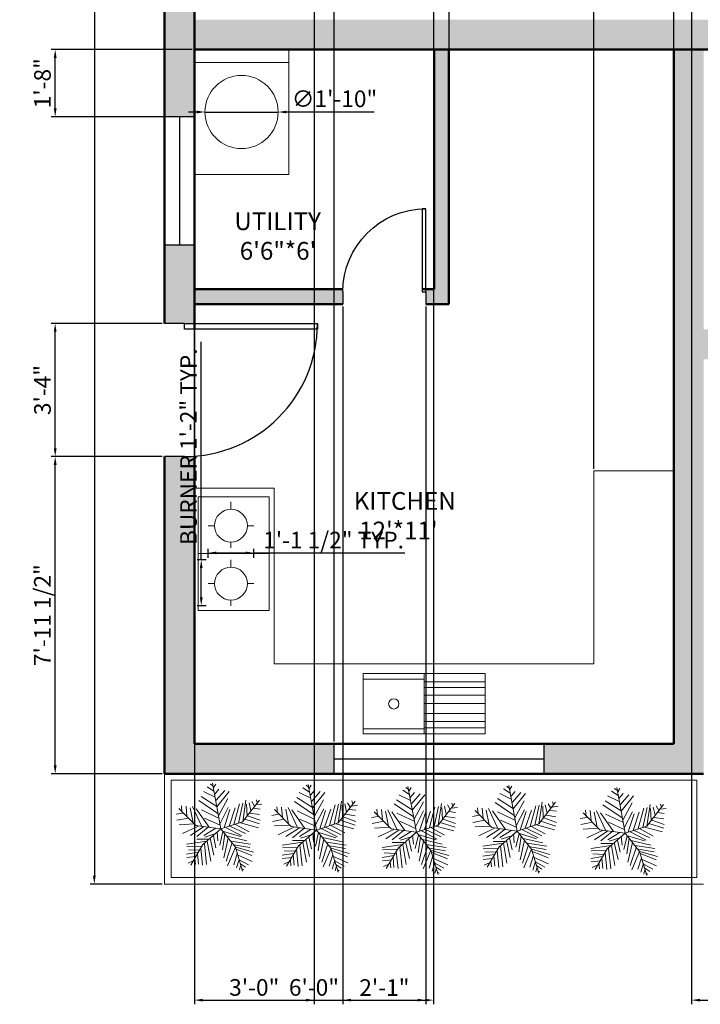
# Model space of a CAD drawing. Units: inches. Extents: x 2152 to 2718, y 1095 to 1798.
# Tile 1 of 5: x 2152 to 2356, y 1098 to 1394. Entities that reach past the tile are written whole.
import ezdxf

# ---------------------------------------------------------------- set-up
doc = ezdxf.new("R2010")
doc.units = ezdxf.units.IN
for name, color, linetype, lineweight in [('A-ANNO-DIMS', 130, 'Continuous', 18), ('A-AREA-IDEN', 130, 'Continuous', 25), ('A-EQPM', 10, 'Continuous', 18), ('A-FLOR-CASE', 10, 'Continuous', 20), ('A-FLOR-FIXT', 10, 'Continuous', 18), ('A-FLOR-STRS', 7, 'Continuous', 25), ('A-WALL-PATT', 210, 'Continuous', 13), ('DOOR', 160, 'Continuous', 25), ('L-PLNT-BEDS', 80, 'Continuous', 18), ('TREE', 80, 'Continuous', 13), ('WALL', 7, 'Continuous', 50), ('WIND', 140, 'Continuous', 25)]:
    doc.layers.add(name, color=color, linetype=linetype, lineweight=lineweight)
doc.styles.get("Standard").update_dxf_attribs({"font": 'arial.ttf'})
doc.dimstyles.new('ISO-25', dxfattribs={"dimtxt": 5, "dimasz": 2.5, "dimexe": 1.25, "dimexo": 0.625, "dimtad": 1, "dimdec": 0, "dimlunit": 4, "dimtxsty": 'Standard', "dimcen": 2.5, "dimadec": 0, "dimazin": 0, "dimtfac": 1, "dimtdec": 0, "dimtmove": 0, "dimatfit": 3, "dimfxl": 1, "dimarcsym": 0})

# ---------------------------------------------------------------- blocks, each defined once
blk = doc.blocks.new('*U6')
for p, q in [((-8.737, 47.138), (-17.069, 52.711)), ((-10.186, 53.64), (-13.084, 55.962)), ((0, 0), (-10.5, 57)), ((-9.099, 51.782), (-6.563, 55.962)), ((-7.65, 43.423), (-2.578, 49.46)), ((-5.114, 28.097), (-24.676, 40.636)), ((-7.288, 39.707), (-21.778, 46.673)), ((-5.839, 35.992), (4.667, 48.067)), ((-5.114, 27.632), (10.463, 46.673)), ((-2.941, 16.486), (8.652, 37.85)), ((-31.5, 4.5), (-52.5, 25.5)), ((-48.585, 21.131), (-49.309, 29.026)), ((-43.513, 28.561), (-42.427, 15.558)), ((-38.442, 26.239), (-34.819, 7.663)), ((-35.544, 28.097), (-24.314, 3.947)), ((-14.533, 2.09), (-30.834, 25.31)), ((-3.665, 19.273), (-27.574, 35.527)), ((-1.129, 6.734), (9.014, 26.704)), ((10.101, 3.483), (17.708, 26.239)), ((16.259, 5.805), (23.142, 31.348)), ((22.055, 7.198), (27.489, 32.277)), ((27, 9), (48, 36)), ((27.127, 9.056), (31.112, 35.992)), ((31.836, 30.883), (32.561, 16.486)), ((35.096, 32.741), (37.27, 22.524)), ((38.719, 34.134), (41.979, 28.561)), ((40.53, 25.775), (48.862, 24.846)), ((43.791, 29.954), (51.036, 30.883)), ((44.153, 36.456), (45.239, 32.741)), ((-47.498, 19.737), (-55.83, 18.344)), ((-40.615, 13.7), (-55.105, 10.913)), ((-24.314, 23.917), (-2.941, 13.7)), ((-20.691, 13.7), (-1.129, 4.876)), ((3.942, 1.625), (11.187, 24.381)), ((29.662, 12.307), (48.137, 6.269)), ((33.285, 16.486), (48.862, 10.913)), ((36.183, 19.737), (48.137, 17.88)), ((-33.37, 6.269), (-52.207, 5.34)), ((-28.299, 3.483), (-47.86, -5.805)), ((-21.416, 3.018), (-38.079, -8.128)), ((0, 0), (-31.5, 4.5)), ((-15.982, 2.09), (-30.11, -9.521)), ((0, 0), (-22.5, -19.5)), ((-6.563, 1.161), (-21.416, -8.128)), ((0, 0), (27, 9)), ((0, 0), (18, -22.5)), ((6.478, 1.625), (26.04, -8.592)), ((11.187, 3.483), (30.749, -5.805)), ((18.07, 5.805), (35.096, -3.483)), ((24.229, 7.663), (46.688, 1.625)), ((-6.563, -5.805), (-19.967, -9.985)), ((-13.446, -11.378), (-8.737, -32.741)), ((-9.461, -8.592), (-6.201, -23.453)), ((-4.752, -3.483), (-3.665, -14.629)), ((2.493, -3.019), (-1.491, -20.202)), ((1.769, -2.555), (24.229, -9.521)), ((5.029, -6.27), (2.131, -25.775)), ((9.014, -11.378), (3.58, -35.992)), ((7.565, -9.056), (32.198, -14.629)), ((-17.431, -15.094), (-42.789, -18.809)), ((-24.314, -21.596), (-42.427, -22.06)), ((-22.5, -19.5), (-37.5, -45)), ((-15.257, -12.772), (-30.11, -12.772)), ((-25.038, -23.918), (-22.865, -45.281)), ((-20.691, -18.345), (-17.793, -44.352)), ((-17.069, -15.094), (-12.721, -40.172)), ((14.085, -16.951), (6.478, -40.172)), ((18.07, -22.524), (8.289, -45.745)), ((12.274, -15.094), (36.907, -18.809)), ((16.259, -19.738), (36.183, -22.989)), ((18, -22.5), (27, -52.5)), ((18.433, -22.524), (40.53, -29.026)), ((-28.299, -29.026), (-42.789, -31.348)), ((-30.834, -34.135), (-42.427, -35.528)), ((-26.849, -26.24), (-40.253, -25.775)), ((-29.023, -30.884), (-27.936, -43.887)), ((20.244, -30.419), (15.897, -44.816)), ((19.157, -25.311), (38.719, -33.206)), ((21.331, -32.741), (39.081, -40.636)), ((-34.457, -39.708), (-40.978, -42.494)), ((-32.646, -36.921), (-31.921, -44.352)), ((22.78, -37.85), (19.519, -48.532)), ((22.78, -38.314), (34.372, -44.816)), ((24.591, -45.745), (23.142, -50.854)), ((24.591, -43.423), (30.749, -47.603)), ((26.764, -49.925), (28.213, -50.854))]:
    blk.add_line(p, q)
blk = doc.blocks.new('*U2')
for p, q in [((0, 0), (0, -6)), ((40, 0), (40, -6))]:
    blk.add_line(p, q)
blk.add_lwpolyline([(0, 0), (0, 40), (1.75, 40), (1.75, 0)], close=True)
blk.add_arc((0, 0), 40, 0, 90)
blk = doc.blocks.new('*D14')
at = {"layer": 'A-ANNO-DIMS', "color": 0, "lineweight": -2, "transparency": 16777216}
for p, q in [((2194.43, 1746.37), (2172.77, 1746.37)), ((2174.02, 1743.87), (2174.02, 1136.72)), ((2194.43, 1134.22), (2172.77, 1134.22))]:
    blk.add_line(p, q, dxfattribs=at)
at = {"layer": 'A-ANNO-DIMS', "color": 0, "transparency": 16777216}
for points in [[(2173.6, 1743.87), (2174.43, 1743.87), (2174.02, 1746.37)], [(2173.6, 1136.72), (2174.43, 1136.72), (2174.02, 1134.22)]]:
    blk.add_solid(points, dxfattribs=at)
at = {"layer": 'Defpoints', "color": 0, "transparency": 16777216}
for p in [(2195.06, 1746.37), (2174.02, 1134.22), (2195.06, 1134.22)]:
    blk.add_point(p, dxfattribs=at)
at = {"layer": 'A-ANNO-DIMS', "color": 0, "transparency": 16777216, "insert": (2170.84, 1440.29), "char_height": 5, "attachment_point": 5, "rotation": 90}
blk.add_mtext("51'", dxfattribs=at)
blk = doc.blocks.new('WIN-WIDE')
blk.add_line((0, 4.5), (63.07, 4.5))
blk.add_lwpolyline([(0, 9), (63.07, 9), (63.07, 0), (0, 0)], close=True)
blk = doc.blocks.new('WIN-NARROW')
blk.add_line((0, 4.5), (38.45, 4.5))
blk.add_lwpolyline([(0, 0), (38.45, 0), (38.45, 9), (0, 9)], close=True)
blk = doc.blocks.new('COOKTOP-BURNER')
for p, q in [((6.87, 11.59), (6.87, 13.8)), ((1.92, 6.64), (0, 6.64)), ((11.82, 6.64), (13.74, 6.64)), ((6.87, 1.69), (6.87, 0))]:
    blk.add_line(p, q)
blk.add_circle((6.87, 6.64), 4.95)
blk = doc.blocks.new('*D32')
at = {"layer": 'A-ANNO-DIMS', "color": 0, "lineweight": -2, "transparency": 16777216}
for p, q in [((2206.13, 1231.61), (2206.13, 1297.05)), ((2207.58, 1231.61), (2204.88, 1231.61)), ((2206.13, 1220.32), (2206.13, 1229.11)), ((2207.58, 1217.82), (2204.88, 1217.82))]:
    blk.add_line(p, q, dxfattribs=at)
at = {"layer": 'A-ANNO-DIMS', "color": 0, "transparency": 16777216}
for points in [[(2205.71, 1229.11), (2206.55, 1229.11), (2206.13, 1231.61)], [(2205.71, 1220.32), (2206.55, 1220.32), (2206.13, 1217.82)]]:
    blk.add_solid(points, dxfattribs=at)
at = {"layer": 'Defpoints', "color": 0, "transparency": 16777216}
for p in [(2206.13, 1231.61), (2208.2, 1231.61), (2208.2, 1217.82)]:
    blk.add_point(p, dxfattribs=at)
at = {"layer": 'A-ANNO-DIMS', "color": 0, "transparency": 16777216, "insert": (2202.95, 1265.58), "char_height": 5, "attachment_point": 5, "rotation": 90}
blk.add_mtext('BURNER 1\'-2" TYP.', dxfattribs=at)
blk = doc.blocks.new('*D33')
at = {"layer": 'A-ANNO-DIMS', "color": 0, "lineweight": -2, "transparency": 16777216}
for p, q in [((2208.2, 1232.24), (2208.2, 1234.93)), ((2210.7, 1233.68), (2219.44, 1233.68)), ((2221.94, 1232.24), (2221.94, 1234.93)), ((2221.94, 1233.68), (2267.34, 1233.68))]:
    blk.add_line(p, q, dxfattribs=at)
at = {"layer": 'A-ANNO-DIMS', "color": 0, "transparency": 16777216}
for points in [[(2210.7, 1234.1), (2210.7, 1233.27), (2208.2, 1233.68)], [(2219.44, 1234.1), (2219.44, 1233.27), (2221.94, 1233.68)]]:
    blk.add_solid(points, dxfattribs=at)
at = {"layer": 'Defpoints', "color": 0, "transparency": 16777216}
for p in [(2221.94, 1233.68), (2208.2, 1231.61), (2221.94, 1231.61)]:
    blk.add_point(p, dxfattribs=at)
at = {"layer": 'A-ANNO-DIMS', "color": 0, "transparency": 16777216, "insert": (2245.89, 1236.89), "char_height": 5, "attachment_point": 5}
blk.add_mtext('1\'-1 1/2" TYP.', dxfattribs=at)
blk = doc.blocks.new('*D36')
at = {"layer": 'A-ANNO-DIMS', "color": 0, "lineweight": -2, "transparency": 16777216}
for p, q in [((2204.06, 1736.74), (2204.06, 1098.09)), ((2275.93, 1736.74), (2275.93, 1098.09)), ((2206.56, 1099.34), (2273.43, 1099.34))]:
    blk.add_line(p, q, dxfattribs=at)
at = {"layer": 'A-ANNO-DIMS', "color": 0, "transparency": 16777216}
for points in [[(2206.56, 1099.75), (2206.56, 1098.92), (2204.06, 1099.34)], [(2273.43, 1099.75), (2273.43, 1098.92), (2275.93, 1099.34)]]:
    blk.add_solid(points, dxfattribs=at)
at = {"layer": 'Defpoints', "color": 0, "transparency": 16777216}
for p in [(2204.06, 1737.37), (2275.93, 1737.37), (2275.93, 1099.34)]:
    blk.add_point(p, dxfattribs=at)
at = {"layer": 'A-ANNO-DIMS', "color": 0, "transparency": 16777216, "insert": (2240, 1102.51), "char_height": 5, "attachment_point": 5}
blk.add_mtext('6\'-0"', dxfattribs=at)
blk = doc.blocks.new('*D41')
at = {"layer": 'A-ANNO-DIMS', "color": 0, "lineweight": -2, "transparency": 16777216}
for p, q in [((2203.43, 1384.87), (2161.01, 1384.87)), ((2162.26, 1367.22), (2162.26, 1382.37)), ((2203.43, 1364.72), (2161.01, 1364.72))]:
    blk.add_line(p, q, dxfattribs=at)
at = {"layer": 'A-ANNO-DIMS', "color": 0, "transparency": 16777216}
for points in [[(2161.84, 1382.37), (2162.68, 1382.37), (2162.26, 1384.87)], [(2161.84, 1367.22), (2162.68, 1367.22), (2162.26, 1364.72)]]:
    blk.add_solid(points, dxfattribs=at)
at = {"layer": 'Defpoints', "color": 0, "transparency": 16777216}
for p in [(2162.26, 1384.87), (2204.06, 1384.87), (2204.06, 1364.72)]:
    blk.add_point(p, dxfattribs=at)
at = {"layer": 'A-ANNO-DIMS', "color": 0, "transparency": 16777216, "insert": (2159.08, 1374.79), "char_height": 5, "attachment_point": 5, "rotation": 90}
blk.add_mtext('1\'-8"', dxfattribs=at)
blk = doc.blocks.new('*D42')
at = {"layer": 'A-ANNO-DIMS', "color": 0, "lineweight": -2, "transparency": 16777216}
for p, q in [((2204.06, 1176.99), (2204.06, 1788.86)), ((2206.56, 1787.61), (2243.52, 1787.61)), ((2246.02, 1176.99), (2246.02, 1788.86))]:
    blk.add_line(p, q, dxfattribs=at)
at = {"layer": 'A-ANNO-DIMS', "color": 0, "transparency": 16777216}
for points in [[(2206.56, 1788.03), (2206.56, 1787.19), (2204.06, 1787.61)], [(2243.52, 1788.03), (2243.52, 1787.19), (2246.02, 1787.61)]]:
    blk.add_solid(points, dxfattribs=at)
at = {"layer": 'Defpoints', "color": 0, "transparency": 16777216}
for p in [(2246.02, 1787.61), (2204.06, 1176.37), (2246.02, 1176.37)]:
    blk.add_point(p, dxfattribs=at)
at = {"layer": 'A-ANNO-DIMS', "color": 0, "transparency": 16777216, "insert": (2225.04, 1790.79), "char_height": 5, "attachment_point": 5}
blk.add_mtext('3\'-6"', dxfattribs=at)
blk = doc.blocks.new('*D45')
at = {"layer": 'A-ANNO-DIMS', "color": 0, "lineweight": -2, "transparency": 16777216}
for p, q in [((2204.06, 1487.74), (2204.06, 1098.09)), ((2240.06, 1487.74), (2240.06, 1098.09)), ((2206.56, 1099.34), (2237.56, 1099.34))]:
    blk.add_line(p, q, dxfattribs=at)
at = {"layer": 'A-ANNO-DIMS', "color": 0, "transparency": 16777216}
for points in [[(2206.56, 1099.75), (2206.56, 1098.92), (2204.06, 1099.34)], [(2237.56, 1099.75), (2237.56, 1098.92), (2240.06, 1099.34)]]:
    blk.add_solid(points, dxfattribs=at)
at = {"layer": 'Defpoints', "color": 0, "transparency": 16777216}
for p in [(2204.06, 1488.37), (2240.06, 1488.37), (2240.06, 1099.34)]:
    blk.add_point(p, dxfattribs=at)
at = {"layer": 'A-ANNO-DIMS', "color": 0, "transparency": 16777216, "insert": (2222.06, 1102.51), "char_height": 5, "attachment_point": 5}
blk.add_mtext('3\'-0"', dxfattribs=at)
blk = doc.blocks.new('*D47')
at = {"layer": 'A-ANNO-DIMS', "color": 0, "lineweight": -2, "transparency": 16777216}
for p, q in [((2248.67, 1307.74), (2248.67, 1098.09)), ((2273.63, 1307.74), (2273.63, 1098.09)), ((2251.17, 1099.34), (2271.13, 1099.34))]:
    blk.add_line(p, q, dxfattribs=at)
at = {"layer": 'A-ANNO-DIMS', "color": 0, "transparency": 16777216}
for points in [[(2251.17, 1099.75), (2251.17, 1098.92), (2248.67, 1099.34)], [(2271.13, 1099.75), (2271.13, 1098.92), (2273.63, 1099.34)]]:
    blk.add_solid(points, dxfattribs=at)
at = {"layer": 'Defpoints', "color": 0, "transparency": 16777216}
for p in [(2248.67, 1308.37), (2273.63, 1308.37), (2273.63, 1099.34)]:
    blk.add_point(p, dxfattribs=at)
at = {"layer": 'A-ANNO-DIMS', "color": 0, "transparency": 16777216, "insert": (2261.15, 1102.47), "char_height": 5, "attachment_point": 5}
blk.add_mtext('2\'-1"', dxfattribs=at)
blk = doc.blocks.new('*D48')
at = {"layer": 'A-ANNO-DIMS', "color": 0, "lineweight": -2, "transparency": 16777216}
for p, q in [((2194.43, 1302.62), (2161.01, 1302.62)), ((2162.26, 1265.12), (2162.26, 1300.12)), ((2194.43, 1262.62), (2161.01, 1262.62))]:
    blk.add_line(p, q, dxfattribs=at)
at = {"layer": 'A-ANNO-DIMS', "color": 0, "transparency": 16777216}
for points in [[(2161.84, 1300.12), (2162.68, 1300.12), (2162.26, 1302.62)], [(2161.84, 1265.12), (2162.68, 1265.12), (2162.26, 1262.62)]]:
    blk.add_solid(points, dxfattribs=at)
at = {"layer": 'Defpoints', "color": 0, "transparency": 16777216}
for p in [(2162.26, 1302.62), (2195.06, 1302.62), (2195.06, 1262.62)]:
    blk.add_point(p, dxfattribs=at)
at = {"layer": 'A-ANNO-DIMS', "color": 0, "transparency": 16777216, "insert": (2159.08, 1282.62), "char_height": 5, "attachment_point": 5, "rotation": 90}
blk.add_mtext('3\'-4"', dxfattribs=at)
blk = doc.blocks.new('*D49')
at = {"layer": 'A-ANNO-DIMS', "color": 0, "lineweight": -2, "transparency": 16777216}
for p, q in [((2194.43, 1262.62), (2161.01, 1262.62)), ((2162.26, 1169.87), (2162.26, 1260.12)), ((2194.43, 1167.37), (2161.01, 1167.37))]:
    blk.add_line(p, q, dxfattribs=at)
at = {"layer": 'A-ANNO-DIMS', "color": 0, "transparency": 16777216}
for points in [[(2161.84, 1260.12), (2162.68, 1260.12), (2162.26, 1262.62)], [(2161.84, 1169.87), (2162.68, 1169.87), (2162.26, 1167.37)]]:
    blk.add_solid(points, dxfattribs=at)
at = {"layer": 'Defpoints', "color": 0, "transparency": 16777216}
for p in [(2162.26, 1262.62), (2195.06, 1262.62), (2195.06, 1167.37)]:
    blk.add_point(p, dxfattribs=at)
at = {"layer": 'A-ANNO-DIMS', "color": 0, "transparency": 16777216, "insert": (2159.05, 1214.99), "char_height": 5, "attachment_point": 5, "rotation": 90}
blk.add_mtext('7\'-11 1/2"', dxfattribs=at)
blk = doc.blocks.new('*D53')
at = {"layer": 'A-ANNO-DIMS', "color": 0, "lineweight": -2, "transparency": 16777216}
for p, q in [((2353.45, 1564.24), (2353.45, 1098.09)), ((2393.45, 1564.24), (2393.45, 1098.09)), ((2355.95, 1099.34), (2390.95, 1099.34))]:
    blk.add_line(p, q, dxfattribs=at)
at = {"layer": 'A-ANNO-DIMS', "color": 0, "transparency": 16777216}
for points in [[(2355.95, 1099.75), (2355.95, 1098.92), (2353.45, 1099.34)], [(2390.95, 1099.75), (2390.95, 1098.92), (2393.45, 1099.34)]]:
    blk.add_solid(points, dxfattribs=at)
at = {"layer": 'Defpoints', "color": 0, "transparency": 16777216}
for p in [(2353.45, 1564.87), (2393.45, 1564.87), (2393.45, 1099.34)]:
    blk.add_point(p, dxfattribs=at)
at = {"layer": 'A-ANNO-DIMS', "color": 0, "transparency": 16777216, "insert": (2373.45, 1102.51), "char_height": 5, "attachment_point": 5}
blk.add_mtext('3\'-4"', dxfattribs=at)
blk = doc.blocks.new('*D68')
at = {"layer": 'A-ANNO-DIMS', "color": 0, "lineweight": -2, "transparency": 16777216}
for p, q in [((2324.06, 1258.93), (2324.06, 1788.86)), ((2326.56, 1787.61), (2345.56, 1787.61)), ((2348.06, 1258.93), (2348.06, 1788.86))]:
    blk.add_line(p, q, dxfattribs=at)
at = {"layer": 'A-ANNO-DIMS', "color": 0, "transparency": 16777216}
for points in [[(2326.56, 1788.03), (2326.56, 1787.19), (2324.06, 1787.61)], [(2345.56, 1788.03), (2345.56, 1787.19), (2348.06, 1787.61)]]:
    blk.add_solid(points, dxfattribs=at)
at = {"layer": 'Defpoints', "color": 0, "transparency": 16777216}
for p in [(2348.06, 1787.61), (2324.06, 1258.3), (2348.06, 1258.3)]:
    blk.add_point(p, dxfattribs=at)
at = {"layer": 'A-ANNO-DIMS', "color": 0, "transparency": 16777216, "insert": (2336.06, 1790.79), "char_height": 5, "attachment_point": 5}
blk.add_mtext('2\'-0"', dxfattribs=at)
blk = doc.blocks.new('*D70')
at = {"layer": 'A-ANNO-DIMS', "color": 0, "lineweight": -2, "transparency": 16777216}
for p, q in [((2204.76, 1366.13), (2202.26, 1366.13)), ((2207.26, 1366.13), (2229.23, 1366.13)), ((2258.1, 1366.13), (2231.73, 1366.13))]:
    blk.add_line(p, q, dxfattribs=at)
at = {"layer": 'A-ANNO-DIMS', "color": 0, "transparency": 16777216}
for points in [[(2204.76, 1366.55), (2204.76, 1365.71), (2207.26, 1366.13)], [(2231.73, 1366.54), (2231.73, 1365.71), (2229.23, 1366.13)]]:
    blk.add_solid(points, dxfattribs=at)
at = {"layer": 'Defpoints', "color": 0, "transparency": 16777216}
for p in [(2207.26, 1366.13), (2229.23, 1366.13)]:
    blk.add_point(p, dxfattribs=at)
at = {"layer": 'A-ANNO-DIMS', "color": 0, "transparency": 16777216, "insert": (2246.17, 1369.45), "char_height": 5, "attachment_point": 5, "rotation": 359.9978}
blk.add_mtext('∅1\'-10"', dxfattribs=at)

msp = doc.modelspace()

# ---------------------------------------------------------------- hatches: boundary and pattern name
at = {"layer": 'A-WALL-PATT'}
h = msp.add_hatch(color=256, dxfattribs=at)
h.dxf.hatch_style = 1
h.paths.add_polyline_path([(2204.06, 1737.37), (2275.93, 1737.37), (2275.93, 1746.37), (2195.06, 1746.37), (2195.06, 1548.16), (2204.06, 1548.16)])
h.paths.add_polyline_path([(2567.46, 1746.37), (2519.79, 1746.37), (2519.79, 1737.37), (2549.06, 1737.37), (2567.46, 1737.37)])
h.paths.add_polyline_path([(2526.56, 1706.63), (2526.56, 1737.37), (2522.06, 1737.37), (2522.06, 1614.04), (2526.56, 1614.04), (2526.56, 1660.87)])
h.paths.add_polyline_path([(2477.06, 1737.37), (2472.56, 1737.37), (2472.56, 1653.37), (2430.09, 1653.37), (2430.09, 1648.87), (2472.56, 1648.87), (2472.56, 1569.37), (2400.56, 1569.37), (2400.56, 1573.72), (2399.94, 1573.72), (2396.06, 1573.72), (2396.06, 1569.37), (2393.45, 1569.37), (2393.45, 1564.87), (2477.06, 1564.87), (2477.06, 1648.87)])
h.paths.add_polyline_path([(2400.56, 1737.37), (2396.06, 1737.37), (2396.06, 1599.61), (2400.56, 1599.61), (2400.56, 1648.87), (2402.42, 1648.87), (2402.42, 1653.37), (2400.56, 1653.37)], flags=17)
h.paths.add_polyline_path([(2353.45, 1569.37), (2204.06, 1569.37), (2204.06, 1564.87), (2353.45, 1564.87)])
h.paths.add_polyline_path([(2280.56, 1492.87), (2221.07, 1492.87), (2221.07, 1488.37), (2280.56, 1488.37)])
h.paths.add_polyline_path([(2221.07, 1492.87), (2204.06, 1492.87), (2204.06, 1488.37), (2221.07, 1488.37)])
h.paths.add_polyline_path([(2280.56, 1536.59), (2276.9, 1536.59, -0.008622), (2276.06, 1536.6), (2276.06, 1492.87), (2280.56, 1492.87)])
h.paths.add_polyline_path([(2280.56, 1564.87), (2276.06, 1564.87), (2276.06, 1560.98), (2276.9, 1560.98), (2280.56, 1560.98)])
h.paths.add_polyline_path([(2675.06, 1746.37), (2630.54, 1746.37), (2630.54, 1737.37), (2666.06, 1737.37), (2666.06, 1384.87), (2675.06, 1384.87)])
h.paths.add_polyline_path([(2666.06, 1569.37), (2578.28, 1569.37), (2526.56, 1569.37), (2526.56, 1574.04), (2522.06, 1574.04), (2522.06, 1564.87), (2522.06, 1560.6), (2526.56, 1560.6), (2526.56, 1564.87), (2666.06, 1564.87)])
h.paths.add_polyline_path([(2526.56, 1520.6), (2522.06, 1520.6), (2522.06, 1384.87), (2570.2, 1384.87), (2570.2, 1393.87), (2526.56, 1393.87)])
h.paths.add_polyline_path([(2666.06, 1393.87), (2633.28, 1393.87), (2633.28, 1384.87), (2666.06, 1384.87)], flags=17)
h.paths.add_polyline_path([(2522.06, 1393.87), (2306.06, 1393.87), (2280.56, 1393.87), (2280.56, 1384.87), (2301.56, 1384.87), (2522.06, 1384.87)])
h.paths.add_polyline_path([(2280.56, 1393.87), (2204.06, 1393.87), (2204.06, 1384.87), (2232.43, 1384.87), (2280.56, 1384.87)])
h.paths.add_polyline_path([(2204.06, 1509.71), (2195.06, 1509.71), (2195.06, 1364.72), (2204.06, 1364.72), (2204.06, 1384.87)])
h.paths.add_polyline_path([(2204.06, 1326.27), (2195.06, 1326.27), (2195.06, 1302.62), (2201.06, 1302.62), (2204.06, 1302.62), (2204.06, 1308.37)])
h.paths.add_polyline_path([(2280.56, 1384.87), (2276.06, 1384.87), (2276.06, 1312.87), (2273.63, 1312.87), (2273.63, 1312.11), (2273.63, 1308.37), (2280.56, 1308.37)])
h.paths.add_polyline_path([(2248.67, 1312.11, -0.007577), (2248.69, 1312.87), (2204.06, 1312.87), (2204.06, 1308.37), (2248.67, 1308.37)])
h.paths.add_polyline_path([(2364.43, 1297.87), (2364.43, 1300.87), (2357.06, 1300.87), (2357.06, 1291.87), (2364.43, 1291.87)])
h.paths.add_polyline_path([(2428.34, 1300.87), (2404.32, 1300.87, -0.01877), (2404.43, 1297.87), (2404.43, 1291.87), (2428.34, 1291.87)])
h.paths.add_polyline_path([(2522.06, 1384.87), (2513.06, 1384.87), (2513.06, 1300.87), (2491.42, 1300.87), (2491.42, 1291.87), (2522.06, 1291.87)])
h.paths.add_polyline_path([(2357.06, 1384.87), (2348.06, 1384.87), (2348.06, 1176.37), (2309.1, 1176.37), (2309.1, 1167.37), (2357.06, 1167.37), (2357.06, 1173.65)])
h.paths.add_polyline_path([(2475.5, 1693.24), (2504.24, 1693.24), (2504.24, 1713.14), (2475.5, 1713.14)], flags=9)
h = msp.add_hatch(color=256, dxfattribs=at)
h.dxf.hatch_style = 1
h.paths.add_polyline_path([(2204.06, 1262.73, -0.01877), (2201.06, 1262.62), (2195.06, 1262.62), (2195.06, 1167.37), (2246.02, 1167.37), (2246.02, 1176.37), (2204.06, 1176.37)])

# ---------------------------------------------------------------- linework, layer by layer
at = {"layer": 'A-EQPM'}
for p, q in [((2204.06, 1380.98), (2232.43, 1380.98)), ((2205.22, 1233.47), (2226.52, 1233.47))]:
    msp.add_line(p, q, dxfattribs=at)
for points in [[(2204.06, 1384.87), (2232.43, 1384.87), (2232.43, 1347.39), (2204.06, 1347.39)], [(2205.22, 1250.53), (2226.52, 1250.53), (2226.52, 1216.41), (2205.22, 1216.41)]]:
    msp.add_lwpolyline(points, close=True, dxfattribs=at)
msp.add_circle((2218.24, 1366.13), 10.99, dxfattribs=at)
at = {"layer": 'A-FLOR-CASE'}
for p, q in [((2348.06, 1258.3), (2324.06, 1258.3)), ((2324.06, 1258.3), (2324.06, 1200.37)), ((2204.06, 1253.16), (2228.06, 1253.16)), ((2228.06, 1253.16), (2228.06, 1200.37)), ((2228.06, 1200.37), (2324.06, 1200.37))]:
    msp.add_line(p, q, dxfattribs=at)
at = {"layer": 'A-FLOR-FIXT'}
for p, q in [((2273.13, 1179.3), (2273.13, 1197.51)), ((2273.13, 1194.93), (2291.47, 1194.93)), ((2273.13, 1193.25), (2291.47, 1193.25)), ((2273.13, 1190.97), (2291.47, 1190.97)), ((2273.13, 1188.44), (2291.47, 1188.44)), ((2273.13, 1185.44), (2291.47, 1185.44)), ((2273.13, 1183.03), (2291.47, 1183.03)), ((2273.13, 1181.11), (2291.47, 1181.11))]:
    msp.add_line(p, q, dxfattribs=at)
for points in [[(2254.79, 1197.51), (2291.47, 1197.51), (2291.47, 1179.3), (2254.79, 1179.3)], [(2254.79, 1195.77), (2273.13, 1195.77), (2273.13, 1180.87), (2254.79, 1180.87)]]:
    msp.add_lwpolyline(points, close=True, dxfattribs=at)
msp.add_circle((2263.96, 1188.32), 1.54, dxfattribs=at)
at = {"layer": 'A-FLOR-STRS'}
msp.add_line((2280.56, 1429.87), (2280.56, 1384.87), dxfattribs=at)
at = {"layer": 'L-PLNT-BEDS'}
for p, q in [((2195.06, 1167.37), (2195.06, 1134.22)), ((2197.06, 1165.37), (2197.06, 1136.22)), ((2197.06, 1165.37), (2355.06, 1165.37)), ((2355.06, 1136.22), (2355.06, 1165.37)), ((2197.06, 1136.22), (2355.06, 1136.22)), ((2195.06, 1134.22), (2357.06, 1134.22))]:
    msp.add_line(p, q, dxfattribs=at)
at = {"layer": 'WALL'}
for p, q in [((2195.06, 1302.62), (2195.06, 1746.37)), ((2204.06, 1300.87), (2204.06, 1737.37)), ((2301.56, 1384.87), (2204.06, 1384.87)), ((2204.06, 1384.87), (2204.06, 1312.87)), ((2276.06, 1312.87), (2276.06, 1384.87)), ((2280.56, 1308.37), (2280.56, 1384.87)), ((2522.06, 1384.87), (2301.56, 1384.87)), ((2348.06, 1176.37), (2348.06, 1384.87)), ((2204.06, 1312.87), (2248.69, 1312.87)), ((2204.06, 1312.87), (2248.69, 1312.87)), ((2272.54, 1312.87), (2276.06, 1312.87)), ((2272.54, 1312.87), (2276.06, 1312.87)), ((2195.06, 1308.37), (2195.06, 1302.62)), ((2204.06, 1308.37), (2248.67, 1308.37)), ((2204.06, 1308.37), (2204.06, 1300.87)), ((2273.63, 1308.37), (2280.56, 1308.37)), ((2195.06, 1206.37), (2195.06, 1262.62)), ((2195.06, 1262.62), (2195.06, 1167.37)), ((2204.06, 1215.37), (2204.06, 1262.73)), ((2204.06, 1262.73), (2204.06, 1176.37)), ((2204.06, 1176.37), (2348.06, 1176.37)), ((2195.06, 1167.37), (2357.06, 1167.37))]:
    msp.add_line(p, q, dxfattribs=at)

# ---------------------------------------------------------------- block references
at = {"layer": 'A-EQPM'}
for p in [(2208.2, 1235.23), (2208.2, 1217.81)]:
    msp.add_blockref('COOKTOP-BURNER', p, dxfattribs=at)
at = {"layer": 'DOOR', "xscale": -0.6239446097208851, "yscale": 0.6239446097208851, "zscale": 0.6239446097208851}
msp.add_blockref('*U2', (2273.63, 1312.11), dxfattribs=at)
at = {"layer": 'DOOR', "rotation": 270}
msp.add_blockref('*U2', (2201.06, 1302.62), dxfattribs=at)
at = {"layer": 'TREE', "xscale": 0.2409617007831742, "yscale": 0.2409617007831742, "zscale": 0.2409617007831742}
for p in [(2212.05, 1150.75), (2240.77, 1150.42), (2270.77, 1149.76), (2301.04, 1150.12), (2333.47, 1149.46)]:
    msp.add_blockref('*U6', p, dxfattribs=at)
at = {"layer": 'WIND', "rotation": 270.0000000000007}
msp.add_blockref('WIN-NARROW', (2195.06, 1364.72), dxfattribs=at)
at = {"layer": 'WIND'}
msp.add_blockref('WIN-WIDE', (2246.02, 1167.37), dxfattribs=at)

# ---------------------------------------------------------------- texts
at = {"layer": 'A-AREA-IDEN', "char_height": 5.331, "attachment_point": 1}
for s, insert in [('UTILITY\\P 6\'6"*6\'', (2216.07, 1335.98)), ("KITCHEN\\P 12'*11'", (2251.94, 1251.96))]:
    msp.add_mtext_dynamic_manual_height_columns(s, width=138.497, gutter_width=26.66, heights=[0], dxfattribs=dict(at, insert=insert))

# ---------------------------------------------------------------- dimensions: what is measured, and where the dimension line sits
at = {"layer": 'A-ANNO-DIMS'}
for base, p1, p2, picture, middle in [((2246.02, 1787.61), (2204.06, 1176.37), (2246.02, 1176.37), '*D42', (2225.04, 1790.79)), ((2348.06, 1787.61), (2324.06, 1258.3), (2348.06, 1258.3), '*D68', (2336.06, 1790.79)), ((2275.93, 1099.34), (2204.06, 1737.37), (2275.93, 1737.37), '*D36', (2240, 1102.51)), ((2393.45, 1099.34), (2353.45, 1564.87), (2393.45, 1564.87), '*D53', (2373.45, 1102.51)), ((2240.06, 1099.34), (2204.06, 1488.37), (2240.06, 1488.37), '*D45', (2222.06, 1102.51)), ((2273.63, 1099.34), (2248.67, 1308.37), (2273.63, 1308.37), '*D47', (2261.15, 1102.47))]:
    dim = msp.add_linear_dim(base=base, p1=p1, p2=p2, dimstyle='ISO-25', override={"dimdec": 1, "dimlfac": 1, "dimrnd": 0, "dimzin": 1, "dimdsep": 46, "dimlunit": 4, "dimfrac": 2}, dxfattribs=at)
    dim.commit()
    dim.dimension.update_dxf_attribs({"geometry": picture, "text_midpoint": middle})
for base, p1, p2, override, picture, middle in [((2174.02, 1134.22), (2195.06, 1746.37), (2195.06, 1134.22), {"dimclrd": 0, "dimclre": 0, "dimclrt": 0}, '*D14', (2170.84, 1440.29)), ((2162.2592, 1384.8669), (2204.0592, 1364.7166), (2204.0592, 1384.8669), {"dimdec": 1, "dimlfac": 1, "dimrnd": 0, "dimzin": 1, "dimdsep": 46, "dimlunit": 4, "dimfrac": 2}, '*D41', (2159.0814, 1374.7917)), ((2162.26, 1302.62), (2195.06, 1262.62), (2195.06, 1302.62), {"dimdec": 1, "dimlfac": 1, "dimrnd": 0, "dimzin": 1, "dimdsep": 46, "dimlunit": 4, "dimfrac": 2}, '*D48', (2159.08, 1282.62)), ((2162.2592, 1262.6202), (2195.0592, 1167.3669), (2195.0592, 1262.6202), {"dimdec": 1, "dimlfac": 1, "dimrnd": 0, "dimzin": 1, "dimdsep": 46, "dimlunit": 4, "dimfrac": 2}, '*D49', (2159.049, 1214.9935))]:
    dim = msp.add_linear_dim(base=base, p1=p1, p2=p2, angle=90, dimstyle='ISO-25', override=override, dxfattribs=at)
    dim.commit()
    dim.dimension.update_dxf_attribs({"geometry": picture, "text_midpoint": middle})
dim = msp.add_diameter_dim_2p(p1=(2207.26, 1366.13), p2=(2229.23, 1366.13), dimstyle='ISO-25', override={"dimdec": 1, "dimlfac": 1, "dimrnd": 0, "dimzin": 1, "dimdsep": 46, "dimlunit": 4, "dimfrac": 2}, dxfattribs=at)
dim.commit()
dim.dimension.update_dxf_attribs({"geometry": '*D70', "text_midpoint": (2246.17, 1366.13), "dimtype": 163})
dim = msp.add_linear_dim(base=(2206.13, 1231.61), p1=(2208.2, 1217.82), p2=(2208.2, 1231.61), angle=90, text='BURNER <> TYP.', dimstyle='ISO-25', override={"dimdec": 1, "dimlfac": 1, "dimrnd": 0, "dimzin": 1, "dimdsep": 46, "dimlunit": 4, "dimfrac": 2}, dxfattribs=at)
dim.commit()
dim.dimension.update_dxf_attribs({"geometry": '*D32', "text_midpoint": (2202.95, 1265.58)})
dim = msp.add_linear_dim(base=(2221.94, 1233.68), p1=(2208.2, 1231.61), p2=(2221.94, 1231.61), text='<> TYP.', dimstyle='ISO-25', override={"dimdec": 1, "dimlfac": 1, "dimrnd": 0, "dimzin": 1, "dimdsep": 46, "dimlunit": 4, "dimfrac": 2}, dxfattribs=at)
dim.commit()
dim.dimension.update_dxf_attribs({"geometry": '*D33', "text_midpoint": (2245.89, 1236.89)})

doc.saveas('drawing.dxf')
